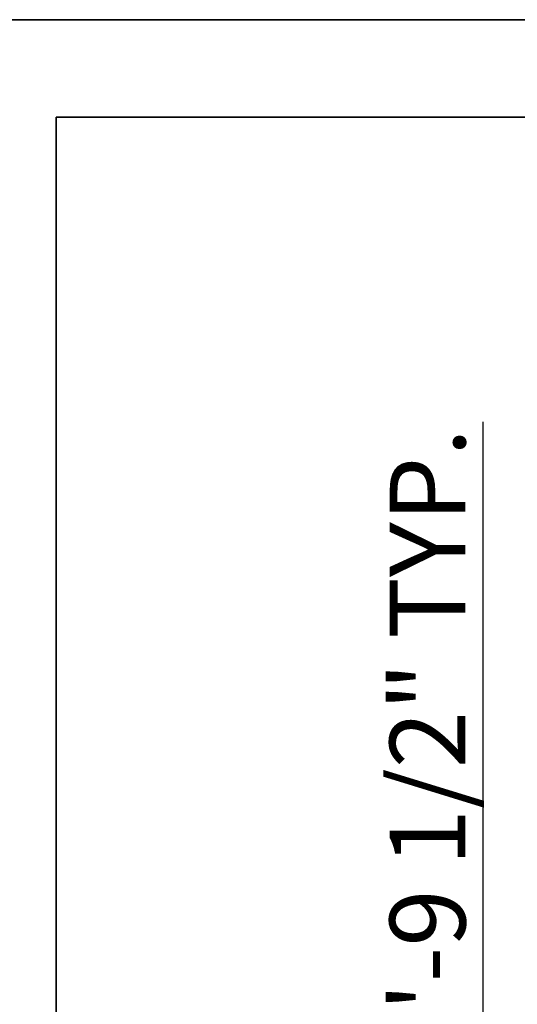
# Model space of a CAD drawing. Units: inches. Extents: x 1484 to 2008, y 1843 to 2590.
# Tile 12 of 21: x 1756 to 1802, y 2126 to 2217. Entities that reach past the tile are written whole.
import ezdxf

# ---------------------------------------------------------------- set-up
doc = ezdxf.new("R2010")
doc.units = ezdxf.units.IN
doc.layers.add('A-ANNO-DIMS', color=2, linetype='Continuous', lineweight=18)
doc.layers.add('A-WALL', color=7, linetype='Continuous', lineweight=35)
doc.styles.get("Standard").update_dxf_attribs({"font": 'arial.ttf'})
doc.dimstyles.new('ISO-25', dxfattribs={"dimtxt": 7, "dimasz": 2.5, "dimexe": 1.25, "dimexo": 0.625, "dimtad": 1, "dimdec": 0, "dimlunit": 3, "dimtxsty": 'Standard', "dimcen": 2.5, "dimadec": 0, "dimazin": 0, "dimtfac": 1, "dimtdec": 0, "dimtmove": 0, "dimatfit": 3, "dimfxl": 1, "dimarcsym": 0})

# ---------------------------------------------------------------- blocks, each defined once
blk = doc.blocks.new('*D2')
at = {"layer": 'A-ANNO-DIMS', "color": 0, "lineweight": -2, "transparency": 16777216}
for p, q in [((1602.92, 2217.928), (1602.92, 2236.385)), ((1899.92, 2217.928), (1899.92, 2236.385)), ((1605.42, 2235.135), (1897.42, 2235.135))]:
    blk.add_line(p, q, dxfattribs=at)
at = {"layer": 'A-ANNO-DIMS', "color": 0, "transparency": 16777216}
for points in [[(1605.42, 2235.552), (1605.42, 2234.719), (1602.92, 2235.135)], [(1897.42, 2235.552), (1897.42, 2234.719), (1899.92, 2235.135)]]:
    blk.add_solid(points, dxfattribs=at)
at = {"layer": 'Defpoints', "color": 0, "transparency": 16777216}
for p in [(1899.92, 2235.135), (1602.92, 2217.303), (1899.92, 2217.303)]:
    blk.add_point(p, dxfattribs=at)
at = {"layer": 'A-ANNO-DIMS', "color": 0, "transparency": 16777216, "insert": (1750.407, 2239.334), "char_height": 7, "attachment_point": 5}
blk.add_mtext('24\'-9"', dxfattribs=at)
blk = doc.blocks.new('*D12')
at = {"layer": 'A-ANNO-DIMS', "color": 0, "lineweight": -2, "transparency": 16777216}
for p, q in [((1798.407, 2117.29), (1798.407, 2180.139)), ((1793.295, 2117.29), (1799.657, 2117.29)), ((1798.407, 2086.463), (1798.407, 2114.79)), ((1793.295, 2083.963), (1799.657, 2083.963))]:
    blk.add_line(p, q, dxfattribs=at)
at = {"layer": 'A-ANNO-DIMS', "color": 0, "transparency": 16777216}
for points in [[(1797.99, 2114.79), (1798.824, 2114.79), (1798.407, 2117.29)], [(1797.99, 2086.463), (1798.824, 2086.463), (1798.407, 2083.963)]]:
    blk.add_solid(points, dxfattribs=at)
at = {"layer": 'Defpoints', "color": 0, "transparency": 16777216}
for p in [(1792.67, 2117.29), (1798.407, 2117.29), (1792.67, 2083.963)]:
    blk.add_point(p, dxfattribs=at)
at = {"layer": 'A-ANNO-DIMS', "color": 0, "transparency": 16777216, "insert": (1794.163, 2149.965), "char_height": 7, "attachment_point": 5, "rotation": 90}
blk.add_mtext('2\'-9 1/2" TYP.', dxfattribs=at)
blk = doc.blocks.new('*D38')
at = {"layer": 'A-ANNO-DIMS', "color": 0, "lineweight": -2, "transparency": 16777216}
for p, q in [((1747.426, 2141.928), (1747.426, 2277.725)), ((1754.42, 2141.928), (1754.42, 2277.725)), ((1749.926, 2276.475), (1751.92, 2276.475)), ((1754.42, 2276.475), (1776.777, 2276.475))]:
    blk.add_line(p, q, dxfattribs=at)
at = {"layer": 'A-ANNO-DIMS', "color": 0, "transparency": 16777216}
for points in [[(1749.926, 2276.891), (1749.926, 2276.058), (1747.426, 2276.475)], [(1751.92, 2276.891), (1751.92, 2276.058), (1754.42, 2276.475)]]:
    blk.add_solid(points, dxfattribs=at)
at = {"layer": 'Defpoints', "color": 0, "transparency": 16777216}
for p in [(1754.42, 2276.475), (1747.426, 2141.303), (1754.42, 2141.303)]:
    blk.add_point(p, dxfattribs=at)
at = {"layer": 'A-ANNO-DIMS', "color": 0, "transparency": 16777216, "insert": (1766.849, 2280.674), "char_height": 7, "attachment_point": 5}
blk.add_mtext('0\'-7"', dxfattribs=at)

msp = doc.modelspace()

# ---------------------------------------------------------------- linework, layer by layer
at = {"layer": 'A-WALL'}
for p, q in [((1602.92, 2217.303), (1899.92, 2217.303)), ((1602.92, 2217.303), (1899.92, 2217.303)), ((1758.92, 2208.303), (1758.92, 2115.666)), ((1758.92, 2208.303), (1890.92, 2208.303))]:
    msp.add_line(p, q, dxfattribs=at)

# ---------------------------------------------------------------- dimensions: what is measured, and where the dimension line sits
at = {"layer": 'A-ANNO-DIMS'}
dim = msp.add_linear_dim(base=(1754.42, 2276.475), p1=(1747.426, 2141.303), p2=(1754.42, 2141.303), dimstyle='ISO-25', override={"dimdec": 1, "dimlfac": 1, "dimrnd": 0, "dimzin": 1, "dimdsep": 46, "dimlunit": 4, "dimfrac": 2}, dxfattribs=at)
dim.commit()
dim.dimension.update_dxf_attribs({"geometry": '*D38', "text_midpoint": (1766.849, 2280.674)})
dim = msp.add_linear_dim(base=(1899.92, 2235.135), p1=(1602.92, 2217.303), p2=(1899.92, 2217.303), dimstyle='ISO-25', override={"dimclrd": 0, "dimclre": 0, "dimclrt": 0}, dxfattribs=at)
dim.commit()
dim.dimension.update_dxf_attribs({"geometry": '*D2', "text_midpoint": (1750.407, 2235.135), "dimtype": 160})
dim = msp.add_linear_dim(base=(1798.407, 2117.29), p1=(1792.67, 2083.963), p2=(1792.67, 2117.29), angle=90, text='<> TYP.', dimstyle='ISO-25', override={"dimdec": 1, "dimlfac": 1, "dimrnd": 0, "dimzin": 1, "dimdsep": 46, "dimlunit": 4, "dimfrac": 2}, dxfattribs=at)
dim.commit()
dim.dimension.update_dxf_attribs({"geometry": '*D12', "text_midpoint": (1794.163, 2149.965)})

doc.saveas('drawing.dxf')
